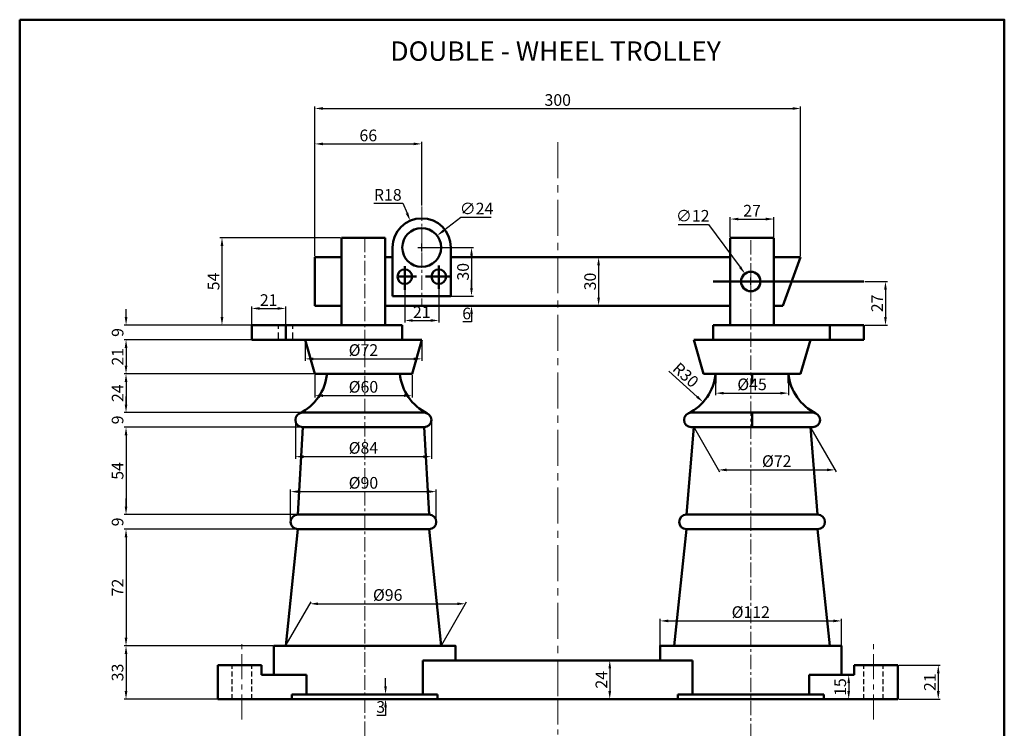
# Model space of a CAD drawing. Units: millimetres. Extents: x -25 to 583, y -116 to 549.
# Tile 2 of 2: x -25 to 583, y 111 to 549. Entities that reach past the tile are written whole.
import ezdxf

# ---------------------------------------------------------------- set-up
doc = ezdxf.new("R2010")
doc.units = ezdxf.units.MM
doc.header["$LTSCALE"] = 0.7
doc.linetypes.add('CENTER', pattern=[50.8, 31.75, -6.35, 6.35, -6.35])
doc.linetypes.add('HIDDEN', pattern=[9.525, 6.35, -3.175])
for name, color, linetype, lineweight in [('M-CNTR', 1, 'CENTER', 18), ('M-DIMS', 2, 'Continuous', 25), ('M-HIDN', 6, 'HIDDEN', 25), ('M-OUTL', 7, 'Continuous', 50), ('M-TEXT', 3, 'Continuous', 25), ('M-TTLB', 7, 'Continuous', 50)]:
    doc.layers.add(name, color=color, linetype=linetype, lineweight=lineweight)
doc.styles.get("Standard").update_dxf_attribs({"font": 'arial.ttf'})
doc.dimstyles.new('ISO-25', dxfattribs={"dimtxt": 7.2, "dimasz": 5, "dimexe": 1.25, "dimexo": 0.625, "dimtad": 1, "dimtoh": 1, "dimdec": 0, "dimtxsty": 'Standard', "dimcen": 2.5, "dimadec": 0, "dimazin": 0, "dimtfac": 1, "dimtdec": 0, "dimtofl": 0, "dimtmove": 0, "dimatfit": 3, "dimfxl": 1, "dimarcsym": 0})

# ---------------------------------------------------------------- blocks, each defined once
blk = doc.blocks.new('*D1')
at = {"layer": 'Defpoints', "color": 0, "ltscale": 0.4, "transparency": 16777216}
for p in [(327.7, 401.89), (327.7, 371.89), (332.69, 371.89)]:
    blk.add_point(p, dxfattribs=at)
at = {"layer": 'M-DIMS', "color": 0, "lineweight": -2, "ltscale": 0.4, "transparency": 16777216}
for p, q in [((328.33, 401.89), (333.94, 401.89)), ((332.69, 396.89), (332.69, 376.89)), ((328.33, 371.89), (333.94, 371.89))]:
    blk.add_line(p, q, dxfattribs=at)
at = {"layer": 'M-DIMS', "color": 0, "ltscale": 0.4, "transparency": 16777216}
for points in [[(331.85, 396.89), (333.52, 396.89), (332.69, 401.89)], [(331.85, 376.89), (333.52, 376.89), (332.69, 371.89)]]:
    blk.add_solid(points, dxfattribs=at)
at = {"layer": 'M-DIMS', "color": 0, "ltscale": 0.4, "transparency": 16777216, "insert": (328.38, 386.89), "char_height": 7.2, "attachment_point": 5, "rotation": 90}
blk.add_mtext('30', dxfattribs=at)
blk = doc.blocks.new('*D2')
at = {"layer": 'Defpoints', "color": 0, "ltscale": 0.4, "transparency": 16777216}
for p in [(250.43, 187.83), (139.45, 161.89), (235.45, 161.89)]:
    blk.add_point(p, dxfattribs=at)
at = {"layer": 'M-DIMS', "color": 0, "lineweight": -2, "ltscale": 0.4, "transparency": 16777216}
for p, q in [((139.81, 162.51), (155.15, 189.08)), ((235.81, 162.51), (251.15, 189.08)), ((159.43, 187.83), (245.43, 187.83))]:
    blk.add_line(p, q, dxfattribs=at)
at = {"layer": 'M-DIMS', "color": 0, "ltscale": 0.4, "transparency": 16777216}
for points in [[(159.43, 188.66), (159.43, 187), (154.43, 187.83)], [(245.43, 188.66), (245.43, 187), (250.43, 187.83)]]:
    blk.add_solid(points, dxfattribs=at)
at = {"layer": 'M-DIMS', "color": 0, "ltscale": 0.4, "transparency": 16777216, "insert": (202.43, 192.33), "char_height": 7.2, "attachment_point": 5}
blk.add_mtext('%%C96', dxfattribs=at)
blk = doc.blocks.new('*D3')
at = {"layer": 'Defpoints', "color": 0, "ltscale": 0.4, "transparency": 16777216}
for p in [(232.45, 257.09), (142.45, 238.39), (232.45, 238.39)]:
    blk.add_point(p, dxfattribs=at)
at = {"layer": 'M-DIMS', "color": 0, "lineweight": -2, "ltscale": 0.4, "transparency": 16777216}
for p, q in [((142.45, 239.01), (142.45, 258.34)), ((147.45, 257.09), (227.45, 257.09)), ((232.45, 239.01), (232.45, 258.34))]:
    blk.add_line(p, q, dxfattribs=at)
at = {"layer": 'M-DIMS', "color": 0, "ltscale": 0.4, "transparency": 16777216}
for points in [[(147.45, 257.93), (147.45, 256.26), (142.45, 257.09)], [(227.45, 257.93), (227.45, 256.26), (232.45, 257.09)]]:
    blk.add_solid(points, dxfattribs=at)
at = {"layer": 'M-DIMS', "color": 0, "ltscale": 0.4, "transparency": 16777216, "insert": (187.45, 261.6), "char_height": 7.2, "attachment_point": 5}
blk.add_mtext('%%C90', dxfattribs=at)
blk = doc.blocks.new('*D4')
at = {"layer": 'Defpoints', "color": 0, "ltscale": 0.4, "transparency": 16777216}
for p in [(145.45, 301.39), (229.45, 301.39), (229.45, 278.69)]:
    blk.add_point(p, dxfattribs=at)
at = {"layer": 'M-DIMS', "color": 0, "lineweight": -2, "ltscale": 0.4, "transparency": 16777216}
for p, q in [((145.45, 300.76), (145.45, 277.44)), ((229.45, 300.76), (229.45, 277.44)), ((150.45, 278.69), (224.45, 278.69))]:
    blk.add_line(p, q, dxfattribs=at)
at = {"layer": 'M-DIMS', "color": 0, "ltscale": 0.4, "transparency": 16777216}
for points in [[(150.45, 279.52), (150.45, 277.86), (145.45, 278.69)], [(224.45, 279.52), (224.45, 277.86), (229.45, 278.69)]]:
    blk.add_solid(points, dxfattribs=at)
at = {"layer": 'M-DIMS', "color": 0, "ltscale": 0.4, "transparency": 16777216, "insert": (187.45, 283.19), "char_height": 7.2, "attachment_point": 5}
blk.add_mtext('%%C84', dxfattribs=at)
blk = doc.blocks.new('*D5')
at = {"layer": 'Defpoints', "color": 0, "ltscale": 0.4, "transparency": 16777216}
for p in [(157.45, 329.89), (217.45, 329.89), (217.45, 316.39)]:
    blk.add_point(p, dxfattribs=at)
at = {"layer": 'M-DIMS', "color": 0, "lineweight": -2, "ltscale": 0.4, "transparency": 16777216}
for p, q in [((157.45, 329.26), (157.45, 315.14)), ((217.45, 329.26), (217.45, 315.14)), ((162.45, 316.39), (212.45, 316.39))]:
    blk.add_line(p, q, dxfattribs=at)
at = {"layer": 'M-DIMS', "color": 0, "ltscale": 0.4, "transparency": 16777216}
for points in [[(162.45, 317.22), (162.45, 315.55), (157.45, 316.39)], [(212.45, 317.22), (212.45, 315.55), (217.45, 316.39)]]:
    blk.add_solid(points, dxfattribs=at)
at = {"layer": 'M-DIMS', "color": 0, "ltscale": 0.4, "transparency": 16777216, "insert": (187.45, 320.89), "char_height": 7.2, "attachment_point": 5}
blk.add_mtext('%%C60', dxfattribs=at)
blk = doc.blocks.new('*D6')
at = {"layer": 'Defpoints', "color": 0, "ltscale": 0.4, "transparency": 16777216}
for p in [(151.45, 350.89), (223.45, 350.89), (223.45, 339.1)]:
    blk.add_point(p, dxfattribs=at)
at = {"layer": 'M-DIMS', "color": 0, "lineweight": -2, "ltscale": 0.4, "transparency": 16777216}
for p, q in [((151.45, 350.26), (151.45, 337.85)), ((223.45, 350.26), (223.45, 337.85)), ((156.45, 339.1), (218.45, 339.1))]:
    blk.add_line(p, q, dxfattribs=at)
at = {"layer": 'M-DIMS', "color": 0, "ltscale": 0.4, "transparency": 16777216}
for points in [[(156.45, 339.93), (156.45, 338.27), (151.45, 339.1)], [(218.45, 339.93), (218.45, 338.27), (223.45, 339.1)]]:
    blk.add_solid(points, dxfattribs=at)
at = {"layer": 'M-DIMS', "color": 0, "ltscale": 0.4, "transparency": 16777216, "insert": (187.45, 343.6), "char_height": 7.2, "attachment_point": 5}
blk.add_mtext('%%C72', dxfattribs=at)
blk = doc.blocks.new('*D7')
at = {"layer": 'Defpoints', "color": 0, "ltscale": 0.4, "transparency": 16777216}
for p in [(404.95, 329.89), (449.95, 329.89), (449.95, 317.91)]:
    blk.add_point(p, dxfattribs=at)
at = {"layer": 'M-DIMS', "color": 0, "lineweight": -2, "ltscale": 0.4, "transparency": 16777216}
for p, q in [((404.95, 329.26), (404.95, 316.66)), ((449.95, 329.26), (449.95, 316.66)), ((409.95, 317.91), (444.95, 317.91))]:
    blk.add_line(p, q, dxfattribs=at)
at = {"layer": 'M-DIMS', "color": 0, "ltscale": 0.4, "transparency": 16777216}
for points in [[(409.95, 318.75), (409.95, 317.08), (404.95, 317.91)], [(444.95, 318.75), (444.95, 317.08), (449.95, 317.91)]]:
    blk.add_solid(points, dxfattribs=at)
at = {"layer": 'M-DIMS', "color": 0, "ltscale": 0.4, "transparency": 16777216, "insert": (427.45, 322.41), "char_height": 7.2, "attachment_point": 5}
blk.add_mtext('%%C45', dxfattribs=at)
blk = doc.blocks.new('*D8')
at = {"layer": 'Defpoints', "color": 0, "ltscale": 0.4, "transparency": 16777216}
for p in [(391.45, 296.89), (463.45, 296.89), (478.68, 270.51)]:
    blk.add_point(p, dxfattribs=at)
at = {"layer": 'M-DIMS', "color": 0, "lineweight": -2, "ltscale": 0.4, "transparency": 16777216}
for p, q in [((391.81, 296.26), (407.4, 269.26)), ((463.81, 296.26), (479.4, 269.26)), ((411.68, 270.51), (473.68, 270.51))]:
    blk.add_line(p, q, dxfattribs=at)
at = {"layer": 'M-DIMS', "color": 0, "ltscale": 0.4, "transparency": 16777216}
for points in [[(411.68, 271.34), (411.68, 269.68), (406.68, 270.51)], [(473.68, 271.34), (473.68, 269.68), (478.68, 270.51)]]:
    blk.add_solid(points, dxfattribs=at)
at = {"layer": 'M-DIMS', "color": 0, "ltscale": 0.4, "transparency": 16777216, "insert": (442.68, 275.01), "char_height": 7.2, "attachment_point": 5}
blk.add_mtext('%%C72', dxfattribs=at)
blk = doc.blocks.new('*D9')
at = {"layer": 'Defpoints', "color": 0, "ltscale": 0.4, "transparency": 16777216}
for p in [(132.22, 161.89), (40.84, 128.89), (132.22, 128.89)]:
    blk.add_point(p, dxfattribs=at)
at = {"layer": 'M-DIMS', "color": 0, "lineweight": -2, "ltscale": 0.4, "transparency": 16777216}
for p, q in [((131.6, 161.89), (39.59, 161.89)), ((40.84, 156.89), (40.84, 133.89)), ((131.6, 128.89), (39.59, 128.89))]:
    blk.add_line(p, q, dxfattribs=at)
at = {"layer": 'M-DIMS', "color": 0, "ltscale": 0.4, "transparency": 16777216}
for points in [[(40, 156.89), (41.67, 156.89), (40.84, 161.89)], [(40, 133.89), (41.67, 133.89), (40.84, 128.89)]]:
    blk.add_solid(points, dxfattribs=at)
at = {"layer": 'M-DIMS', "color": 0, "ltscale": 0.4, "transparency": 16777216, "insert": (36.53, 145.39), "char_height": 7.2, "attachment_point": 5, "rotation": 90}
blk.add_mtext('33', dxfattribs=at)
blk = doc.blocks.new('*D10')
at = {"layer": 'Defpoints', "color": 0, "ltscale": 0.4, "transparency": 16777216}
for p in [(158.13, 233.89), (40.84, 161.89), (114.46, 161.89)]:
    blk.add_point(p, dxfattribs=at)
at = {"layer": 'M-DIMS', "color": 0, "lineweight": -2, "ltscale": 0.4, "transparency": 16777216}
for p, q in [((157.5, 233.89), (39.59, 233.89)), ((40.84, 228.89), (40.84, 166.89)), ((113.84, 161.89), (39.59, 161.89))]:
    blk.add_line(p, q, dxfattribs=at)
at = {"layer": 'M-DIMS', "color": 0, "ltscale": 0.4, "transparency": 16777216}
for points in [[(40, 228.89), (41.67, 228.89), (40.84, 233.89)], [(40, 166.89), (41.67, 166.89), (40.84, 161.89)]]:
    blk.add_solid(points, dxfattribs=at)
at = {"layer": 'M-DIMS', "color": 0, "ltscale": 0.4, "transparency": 16777216, "insert": (36.6, 197.89), "char_height": 7.2, "attachment_point": 5, "rotation": 90}
blk.add_mtext('72', dxfattribs=at)
blk = doc.blocks.new('*D11')
at = {"layer": 'Defpoints', "color": 0, "ltscale": 0.4, "transparency": 16777216}
for p in [(146.95, 242.89), (40.84, 233.89), (146.95, 233.89)]:
    blk.add_point(p, dxfattribs=at)
at = {"layer": 'M-DIMS', "color": 0, "lineweight": -2, "ltscale": 0.4, "transparency": 16777216}
for p, q in [((40.84, 247.89), (40.84, 252.89)), ((146.33, 242.89), (39.59, 242.89)), ((146.33, 233.89), (39.59, 233.89)), ((40.84, 228.89), (40.84, 223.89))]:
    blk.add_line(p, q, dxfattribs=at)
at = {"layer": 'M-DIMS', "color": 0, "ltscale": 0.4, "transparency": 16777216}
for points in [[(40, 247.89), (41.67, 247.89), (40.84, 242.89)], [(40, 228.89), (41.67, 228.89), (40.84, 233.89)]]:
    blk.add_solid(points, dxfattribs=at)
at = {"layer": 'M-DIMS', "color": 0, "ltscale": 0.4, "transparency": 16777216, "insert": (36.54, 238.39), "char_height": 7.2, "attachment_point": 5, "rotation": 90}
blk.add_mtext('9', dxfattribs=at)
blk = doc.blocks.new('*D12')
at = {"layer": 'Defpoints', "color": 0, "ltscale": 0.4, "transparency": 16777216}
for p in [(154.98, 296.89), (40.84, 242.89), (154.98, 242.89)]:
    blk.add_point(p, dxfattribs=at)
at = {"layer": 'M-DIMS', "color": 0, "lineweight": -2, "ltscale": 0.4, "transparency": 16777216}
for p, q in [((154.35, 296.89), (39.59, 296.89)), ((40.84, 291.89), (40.84, 247.89)), ((154.35, 242.89), (39.59, 242.89))]:
    blk.add_line(p, q, dxfattribs=at)
at = {"layer": 'M-DIMS', "color": 0, "ltscale": 0.4, "transparency": 16777216}
for points in [[(40, 291.89), (41.67, 291.89), (40.84, 296.89)], [(40, 247.89), (41.67, 247.89), (40.84, 242.89)]]:
    blk.add_solid(points, dxfattribs=at)
at = {"layer": 'M-DIMS', "color": 0, "ltscale": 0.4, "transparency": 16777216, "insert": (36.55, 269.89), "char_height": 7.2, "attachment_point": 5, "rotation": 90}
blk.add_mtext('54', dxfattribs=at)
blk = doc.blocks.new('*D13')
at = {"layer": 'Defpoints', "color": 0, "ltscale": 0.4, "transparency": 16777216}
for p in [(179.78, 305.89), (40.84, 296.89), (179.78, 296.89)]:
    blk.add_point(p, dxfattribs=at)
at = {"layer": 'M-DIMS', "color": 0, "lineweight": -2, "ltscale": 0.4, "transparency": 16777216}
for p, q in [((40.84, 310.89), (40.84, 315.89)), ((179.15, 305.89), (39.59, 305.89)), ((179.15, 296.89), (39.59, 296.89)), ((40.84, 291.89), (40.84, 286.89))]:
    blk.add_line(p, q, dxfattribs=at)
at = {"layer": 'M-DIMS', "color": 0, "ltscale": 0.4, "transparency": 16777216}
for points in [[(40, 310.89), (41.67, 310.89), (40.84, 305.89)], [(40, 291.89), (41.67, 291.89), (40.84, 296.89)]]:
    blk.add_solid(points, dxfattribs=at)
at = {"layer": 'M-DIMS', "color": 0, "ltscale": 0.4, "transparency": 16777216, "insert": (36.54, 301.39), "char_height": 7.2, "attachment_point": 5, "rotation": 90}
blk.add_mtext('9', dxfattribs=at)
blk = doc.blocks.new('*D14')
at = {"layer": 'Defpoints', "color": 0, "ltscale": 0.4, "transparency": 16777216}
for p in [(164.95, 329.89), (40.84, 305.89), (164.95, 305.89)]:
    blk.add_point(p, dxfattribs=at)
at = {"layer": 'M-DIMS', "color": 0, "lineweight": -2, "ltscale": 0.4, "transparency": 16777216}
for p, q in [((164.33, 329.89), (39.59, 329.89)), ((40.84, 324.89), (40.84, 310.89)), ((164.33, 305.89), (39.59, 305.89))]:
    blk.add_line(p, q, dxfattribs=at)
at = {"layer": 'M-DIMS', "color": 0, "ltscale": 0.4, "transparency": 16777216}
for points in [[(40, 324.89), (41.67, 324.89), (40.84, 329.89)], [(40, 310.89), (41.67, 310.89), (40.84, 305.89)]]:
    blk.add_solid(points, dxfattribs=at)
at = {"layer": 'M-DIMS', "color": 0, "ltscale": 0.4, "transparency": 16777216, "insert": (36.6, 317.89), "char_height": 7.2, "attachment_point": 5, "rotation": 90}
blk.add_mtext('24', dxfattribs=at)
blk = doc.blocks.new('*D15')
at = {"layer": 'Defpoints', "color": 0, "ltscale": 0.4, "transparency": 16777216}
for p in [(158.97, 350.89), (40.84, 329.89), (158.97, 329.89)]:
    blk.add_point(p, dxfattribs=at)
at = {"layer": 'M-DIMS', "color": 0, "lineweight": -2, "ltscale": 0.4, "transparency": 16777216}
for p, q in [((158.35, 350.89), (39.59, 350.89)), ((40.84, 345.89), (40.84, 334.89)), ((158.35, 329.89), (39.59, 329.89))]:
    blk.add_line(p, q, dxfattribs=at)
at = {"layer": 'M-DIMS', "color": 0, "ltscale": 0.4, "transparency": 16777216}
for points in [[(40, 345.89), (41.67, 345.89), (40.84, 350.89)], [(40, 334.89), (41.67, 334.89), (40.84, 329.89)]]:
    blk.add_solid(points, dxfattribs=at)
at = {"layer": 'M-DIMS', "color": 0, "ltscale": 0.4, "transparency": 16777216, "insert": (36.6, 340.39), "char_height": 7.2, "attachment_point": 5, "rotation": 90}
blk.add_mtext('21', dxfattribs=at)
blk = doc.blocks.new('*D16')
at = {"layer": 'Defpoints', "color": 0, "ltscale": 0.4, "transparency": 16777216}
for p in [(118.45, 359.89), (40.86, 350.89), (118.45, 350.89)]:
    blk.add_point(p, dxfattribs=at)
at = {"layer": 'M-DIMS', "color": 0, "lineweight": -2, "ltscale": 0.4, "transparency": 16777216}
for p, q in [((40.86, 364.89), (40.86, 369.89)), ((117.83, 359.89), (39.61, 359.89)), ((117.83, 350.89), (39.61, 350.89)), ((40.86, 345.89), (40.86, 340.89))]:
    blk.add_line(p, q, dxfattribs=at)
at = {"layer": 'M-DIMS', "color": 0, "ltscale": 0.4, "transparency": 16777216}
for points in [[(40.03, 364.89), (41.69, 364.89), (40.86, 359.89)], [(40.03, 345.89), (41.69, 345.89), (40.86, 350.89)]]:
    blk.add_solid(points, dxfattribs=at)
at = {"layer": 'M-DIMS', "color": 0, "ltscale": 0.4, "transparency": 16777216, "insert": (36.56, 355.39), "char_height": 7.2, "attachment_point": 5, "rotation": 90}
blk.add_mtext('9', dxfattribs=at)
blk = doc.blocks.new('*D17')
at = {"layer": 'Defpoints', "color": 0, "ltscale": 0.4, "transparency": 16777216}
for p in [(173.95, 413.89), (100.1, 359.89), (173.95, 359.89)]:
    blk.add_point(p, dxfattribs=at)
at = {"layer": 'M-DIMS', "color": 0, "lineweight": -2, "ltscale": 0.4, "transparency": 16777216}
for p, q in [((173.33, 413.89), (98.85, 413.89)), ((100.1, 408.89), (100.1, 364.89)), ((173.33, 359.89), (98.85, 359.89))]:
    blk.add_line(p, q, dxfattribs=at)
at = {"layer": 'M-DIMS', "color": 0, "ltscale": 0.4, "transparency": 16777216}
for points in [[(99.27, 408.89), (100.94, 408.89), (100.1, 413.89)], [(99.27, 364.89), (100.94, 364.89), (100.1, 359.89)]]:
    blk.add_solid(points, dxfattribs=at)
at = {"layer": 'M-DIMS', "color": 0, "ltscale": 0.4, "transparency": 16777216, "insert": (95.82, 386.89), "char_height": 7.2, "attachment_point": 5, "rotation": 90}
blk.add_mtext('54', dxfattribs=at)
blk = doc.blocks.new('*D18')
at = {"layer": 'Defpoints', "color": 0, "ltscale": 0.4, "transparency": 16777216}
for p in [(139.45, 370.24), (118.45, 359.89), (139.45, 359.89)]:
    blk.add_point(p, dxfattribs=at)
at = {"layer": 'M-DIMS', "color": 0, "lineweight": -2, "ltscale": 0.4, "transparency": 16777216}
for p, q in [((118.45, 360.51), (118.45, 371.49)), ((139.45, 360.51), (139.45, 371.49)), ((123.45, 370.24), (134.45, 370.24))]:
    blk.add_line(p, q, dxfattribs=at)
at = {"layer": 'M-DIMS', "color": 0, "ltscale": 0.4, "transparency": 16777216}
for points in [[(123.45, 371.07), (123.45, 369.4), (118.45, 370.24)], [(134.45, 371.07), (134.45, 369.4), (139.45, 370.24)]]:
    blk.add_solid(points, dxfattribs=at)
at = {"layer": 'M-DIMS', "color": 0, "ltscale": 0.4, "transparency": 16777216, "insert": (128.95, 374.48), "char_height": 7.2, "attachment_point": 5}
blk.add_mtext('21', dxfattribs=at)
blk = doc.blocks.new('*D19')
at = {"layer": 'Defpoints', "color": 0, "ltscale": 0.4, "transparency": 16777216}
for p in [(457.45, 493.74), (157.45, 401.89), (457.45, 401.89)]:
    blk.add_point(p, dxfattribs=at)
at = {"layer": 'M-DIMS', "color": 0, "lineweight": -2, "ltscale": 0.4, "transparency": 16777216}
for p, q in [((157.45, 402.51), (157.45, 494.99)), ((162.45, 493.74), (452.45, 493.74)), ((457.45, 402.51), (457.45, 494.99))]:
    blk.add_line(p, q, dxfattribs=at)
at = {"layer": 'M-DIMS', "color": 0, "ltscale": 0.4, "transparency": 16777216}
for points in [[(162.45, 494.57), (162.45, 492.91), (157.45, 493.74)], [(452.45, 494.57), (452.45, 492.91), (457.45, 493.74)]]:
    blk.add_solid(points, dxfattribs=at)
at = {"layer": 'M-DIMS', "color": 0, "ltscale": 0.4, "transparency": 16777216, "insert": (307.45, 498.04), "char_height": 7.2, "attachment_point": 5}
blk.add_mtext('300', dxfattribs=at)
blk = doc.blocks.new('*D20')
at = {"layer": 'Defpoints', "color": 0, "ltscale": 0.4, "transparency": 16777216}
for p in [(223.45, 471.87), (157.45, 448.75), (223.45, 433.22)]:
    blk.add_point(p, dxfattribs=at)
at = {"layer": 'M-DIMS', "color": 0, "lineweight": -2, "ltscale": 0.4, "transparency": 16777216}
for p, q in [((157.45, 449.38), (157.45, 473.12)), ((162.45, 471.87), (218.45, 471.87)), ((223.45, 433.84), (223.45, 473.12))]:
    blk.add_line(p, q, dxfattribs=at)
at = {"layer": 'M-DIMS', "color": 0, "ltscale": 0.4, "transparency": 16777216}
for points in [[(162.45, 472.7), (162.45, 471.03), (157.45, 471.87)], [(218.45, 472.7), (218.45, 471.03), (223.45, 471.87)]]:
    blk.add_solid(points, dxfattribs=at)
at = {"layer": 'M-DIMS', "color": 0, "ltscale": 0.4, "transparency": 16777216, "insert": (190.45, 476.17), "char_height": 7.2, "attachment_point": 5}
blk.add_mtext('66', dxfattribs=at)
blk = doc.blocks.new('*D21')
at = {"layer": 'Defpoints', "color": 0, "ltscale": 0.4, "transparency": 16777216}
for p in [(237.7, 377.89), (237.7, 371.89), (254.2, 371.89)]:
    blk.add_point(p, dxfattribs=at)
at = {"layer": 'M-DIMS', "color": 0, "lineweight": -2, "ltscale": 0.4, "transparency": 16777216}
for p, q in [((254.2, 382.89), (254.2, 387.89)), ((238.33, 377.89), (255.45, 377.89)), ((238.33, 371.89), (255.45, 371.89)), ((254.2, 366.89), (254.2, 361.89)), ((254.2, 361.89), (248.82, 361.89))]:
    blk.add_line(p, q, dxfattribs=at)
at = {"layer": 'M-DIMS', "color": 0, "ltscale": 0.4, "transparency": 16777216}
for points in [[(253.37, 382.89), (255.03, 382.89), (254.2, 377.89)], [(253.37, 366.89), (255.03, 366.89), (254.2, 371.89)]]:
    blk.add_solid(points, dxfattribs=at)
at = {"layer": 'M-DIMS', "color": 0, "ltscale": 0.4, "transparency": 16777216, "insert": (251.2, 366.19), "char_height": 7.2, "attachment_point": 5}
blk.add_mtext('6', dxfattribs=at)
blk = doc.blocks.new('*D22')
at = {"layer": 'Defpoints', "color": 0, "ltscale": 0.4, "transparency": 16777216}
for p in [(223.45, 407.89), (223.45, 377.89), (254.2, 377.89)]:
    blk.add_point(p, dxfattribs=at)
at = {"layer": 'M-DIMS', "color": 0, "lineweight": -2, "ltscale": 0.4, "transparency": 16777216}
for p, q in [((224.08, 407.89), (255.45, 407.89)), ((254.2, 402.89), (254.2, 382.89)), ((224.08, 377.89), (255.45, 377.89))]:
    blk.add_line(p, q, dxfattribs=at)
at = {"layer": 'M-DIMS', "color": 0, "ltscale": 0.4, "transparency": 16777216}
for points in [[(253.37, 402.89), (255.03, 402.89), (254.2, 407.89)], [(253.37, 382.89), (255.03, 382.89), (254.2, 377.89)]]:
    blk.add_solid(points, dxfattribs=at)
at = {"layer": 'M-DIMS', "color": 0, "ltscale": 0.4, "transparency": 16777216, "insert": (249.9, 392.89), "char_height": 7.2, "attachment_point": 5, "rotation": 90}
blk.add_mtext('30', dxfattribs=at)
blk = doc.blocks.new('*D23')
at = {"layer": 'Defpoints', "color": 0, "ltscale": 0.4, "transparency": 16777216}
for p in [(212.95, 389.89), (233.95, 389.89), (233.95, 362.81)]:
    blk.add_point(p, dxfattribs=at)
at = {"layer": 'M-DIMS', "color": 0, "lineweight": -2, "ltscale": 0.4, "transparency": 16777216}
for p, q in [((212.95, 389.26), (212.95, 361.56)), ((233.95, 389.26), (233.95, 361.56)), ((217.95, 362.81), (228.95, 362.81))]:
    blk.add_line(p, q, dxfattribs=at)
at = {"layer": 'M-DIMS', "color": 0, "ltscale": 0.4, "transparency": 16777216}
for points in [[(217.95, 363.64), (217.95, 361.98), (212.95, 362.81)], [(228.95, 363.64), (228.95, 361.98), (233.95, 362.81)]]:
    blk.add_solid(points, dxfattribs=at)
at = {"layer": 'M-DIMS', "color": 0, "ltscale": 0.4, "transparency": 16777216, "insert": (223.45, 367.05), "char_height": 7.2, "attachment_point": 5}
blk.add_mtext('21', dxfattribs=at)
blk = doc.blocks.new('*D24')
at = {"layer": 'Defpoints', "color": 0, "ltscale": 0.4, "transparency": 16777216}
for p in [(232.96, 415.2), (213.94, 400.57)]:
    blk.add_point(p, dxfattribs=at)
at = {"layer": 'M-DIMS', "color": 0, "lineweight": -2, "ltscale": 0.4, "transparency": 16777216}
for p, q in [((247.63, 426.48), (236.93, 418.25)), ((266.37, 426.48), (247.63, 426.48)), ((220.95, 407.89), (225.95, 407.89)), ((223.45, 405.39), (223.45, 410.39))]:
    blk.add_line(p, q, dxfattribs=at)
at = {"layer": 'M-DIMS', "color": 0, "ltscale": 0.4, "transparency": 16777216}
blk.add_solid([(236.42, 418.91), (237.43, 417.59), (232.96, 415.2)], dxfattribs=at)
at = {"layer": 'M-DIMS', "color": 0, "ltscale": 0.4, "transparency": 16777216, "insert": (257.31, 430.98), "char_height": 7.2, "attachment_point": 5}
blk.add_mtext('∅24', dxfattribs=at)
blk = doc.blocks.new('*D25')
at = {"layer": 'Defpoints', "color": 0, "ltscale": 0.4, "transparency": 16777216}
for p in [(216.34, 424.42), (223.45, 407.89)]:
    blk.add_point(p, dxfattribs=at)
at = {"layer": 'M-DIMS', "color": 0, "lineweight": -2, "ltscale": 0.4, "transparency": 16777216}
for p, q in [((193.88, 435.17), (211.72, 435.17)), ((211.72, 435.17), (214.37, 429.02)), ((220.95, 407.89), (225.95, 407.89)), ((223.45, 405.39), (223.45, 410.39))]:
    blk.add_line(p, q, dxfattribs=at)
at = {"layer": 'M-DIMS', "color": 0, "ltscale": 0.4, "transparency": 16777216}
blk.add_solid([(215.13, 429.35), (213.6, 428.69), (216.34, 424.42)], dxfattribs=at)
at = {"layer": 'M-DIMS', "color": 0, "ltscale": 0.4, "transparency": 16777216, "insert": (202.49, 439.47), "char_height": 7.2, "attachment_point": 5}
blk.add_mtext('R18', dxfattribs=at)
blk = doc.blocks.new('*D26')
at = {"layer": 'Defpoints', "color": 0, "ltscale": 0.4, "transparency": 16777216}
for p in [(496.45, 386.89), (496.45, 359.89), (509.86, 359.89)]:
    blk.add_point(p, dxfattribs=at)
at = {"layer": 'M-DIMS', "color": 0, "lineweight": -2, "ltscale": 0.4, "transparency": 16777216}
for p, q in [((497.08, 386.89), (511.11, 386.89)), ((509.86, 381.89), (509.86, 364.89)), ((497.08, 359.89), (511.11, 359.89))]:
    blk.add_line(p, q, dxfattribs=at)
at = {"layer": 'M-DIMS', "color": 0, "ltscale": 0.4, "transparency": 16777216}
for points in [[(509.02, 381.89), (510.69, 381.89), (509.86, 386.89)], [(509.02, 364.89), (510.69, 364.89), (509.86, 359.89)]]:
    blk.add_solid(points, dxfattribs=at)
at = {"layer": 'M-DIMS', "color": 0, "ltscale": 0.4, "transparency": 16777216, "insert": (505.62, 373.39), "char_height": 7.2, "attachment_point": 5, "rotation": 90}
blk.add_mtext('27', dxfattribs=at)
blk = doc.blocks.new('*D27')
at = {"layer": 'Defpoints', "color": 0, "ltscale": 0.4, "transparency": 16777216}
for p in [(440.95, 425.45), (413.95, 413.89), (440.95, 413.89)]:
    blk.add_point(p, dxfattribs=at)
at = {"layer": 'M-DIMS', "color": 0, "lineweight": -2, "ltscale": 0.4, "transparency": 16777216}
for p, q in [((413.95, 414.51), (413.95, 426.7)), ((440.95, 414.51), (440.95, 426.7)), ((418.95, 425.45), (435.95, 425.45))]:
    blk.add_line(p, q, dxfattribs=at)
at = {"layer": 'M-DIMS', "color": 0, "ltscale": 0.4, "transparency": 16777216}
for points in [[(418.95, 426.28), (418.95, 424.62), (413.95, 425.45)], [(435.95, 426.28), (435.95, 424.62), (440.95, 425.45)]]:
    blk.add_solid(points, dxfattribs=at)
at = {"layer": 'M-DIMS', "color": 0, "ltscale": 0.4, "transparency": 16777216, "insert": (427.45, 429.69), "char_height": 7.2, "attachment_point": 5}
blk.add_mtext('27', dxfattribs=at)
blk = doc.blocks.new('*D28')
at = {"layer": 'Defpoints', "color": 0, "ltscale": 0.4, "transparency": 16777216}
for p in [(374.67, 332.79), (397.22, 312.37)]:
    blk.add_point(p, dxfattribs=at)
at = {"layer": 'M-DIMS', "color": 0, "lineweight": -2, "ltscale": 0.4, "transparency": 16777216}
blk.add_line((376.14, 331.45), (393.51, 315.73), dxfattribs=at)
at = {"layer": 'M-DIMS', "color": 0, "ltscale": 0.4, "transparency": 16777216}
blk.add_solid([(394.07, 316.34), (392.96, 315.11), (397.22, 312.37)], dxfattribs=at)
at = {"layer": 'M-DIMS', "color": 0, "ltscale": 0.4, "transparency": 16777216, "insert": (385.86, 328.46), "char_height": 7.2, "attachment_point": 5, "rotation": 317.84948}
blk.add_mtext('R30', dxfattribs=at)
blk = doc.blocks.new('*D29')
at = {"layer": 'Defpoints', "color": 0, "ltscale": 0.4, "transparency": 16777216}
for p in [(423.09, 391.7), (430.27, 382.08)]:
    blk.add_point(p, dxfattribs=at)
at = {"layer": 'M-DIMS', "color": 0, "lineweight": -2, "ltscale": 0.4, "transparency": 16777216}
for p, q in [((381.8, 422.01), (400.5, 422.01)), ((400.5, 422.01), (420.11, 395.7)), ((426.68, 384.39), (426.68, 389.39)), ((424.18, 386.89), (429.18, 386.89))]:
    blk.add_line(p, q, dxfattribs=at)
at = {"layer": 'M-DIMS', "color": 0, "ltscale": 0.4, "transparency": 16777216}
blk.add_solid([(420.77, 396.2), (419.44, 395.21), (423.09, 391.7)], dxfattribs=at)
at = {"layer": 'M-DIMS', "color": 0, "ltscale": 0.4, "transparency": 16777216, "insert": (390.83, 426.51), "char_height": 7.2, "attachment_point": 5}
blk.add_mtext('∅12', dxfattribs=at)
blk = doc.blocks.new('*D30')
at = {"layer": 'Defpoints', "color": 0, "ltscale": 0.4, "transparency": 16777216}
for p in [(482.68, 177.24), (370.68, 161.89), (482.68, 161.89)]:
    blk.add_point(p, dxfattribs=at)
at = {"layer": 'M-DIMS', "color": 0, "lineweight": -2, "ltscale": 0.4, "transparency": 16777216}
for p, q in [((370.68, 162.51), (370.68, 178.49)), ((375.68, 177.24), (477.68, 177.24)), ((482.68, 162.51), (482.68, 178.49))]:
    blk.add_line(p, q, dxfattribs=at)
at = {"layer": 'M-DIMS', "color": 0, "ltscale": 0.4, "transparency": 16777216}
for points in [[(375.68, 178.08), (375.68, 176.41), (370.68, 177.24)], [(477.68, 178.08), (477.68, 176.41), (482.68, 177.24)]]:
    blk.add_solid(points, dxfattribs=at)
at = {"layer": 'M-DIMS', "color": 0, "ltscale": 0.4, "transparency": 16777216, "insert": (426.68, 181.74), "char_height": 7.2, "attachment_point": 5}
blk.add_mtext('%%C112', dxfattribs=at)
blk = doc.blocks.new('*D31')
at = {"layer": 'Defpoints', "color": 0, "ltscale": 0.4, "transparency": 16777216}
for p in [(517.45, 149.89), (517.45, 128.89), (542.46, 128.89)]:
    blk.add_point(p, dxfattribs=at)
at = {"layer": 'M-DIMS', "color": 0, "lineweight": -2, "ltscale": 0.4, "transparency": 16777216}
for p, q in [((518.08, 149.89), (543.71, 149.89)), ((542.46, 144.89), (542.46, 133.89)), ((518.08, 128.89), (543.71, 128.89))]:
    blk.add_line(p, q, dxfattribs=at)
at = {"layer": 'M-DIMS', "color": 0, "ltscale": 0.4, "transparency": 16777216}
for points in [[(541.62, 144.89), (543.29, 144.89), (542.46, 149.89)], [(541.62, 133.89), (543.29, 133.89), (542.46, 128.89)]]:
    blk.add_solid(points, dxfattribs=at)
at = {"layer": 'M-DIMS', "color": 0, "ltscale": 0.4, "transparency": 16777216, "insert": (538.22, 139.39), "char_height": 7.2, "attachment_point": 5, "rotation": 90}
blk.add_mtext('21', dxfattribs=at)
blk = doc.blocks.new('*D32')
at = {"layer": 'Defpoints', "color": 0, "ltscale": 0.7, "transparency": 16777216}
for p in [(486.74, 143.89), (486.74, 128.89), (487.14, 128.89)]:
    blk.add_point(p, dxfattribs=at)
at = {"layer": 'M-DIMS', "color": 0, "lineweight": -2, "ltscale": 0.7, "transparency": 16777216}
for p, q in [((487.36, 143.89), (488.39, 143.89)), ((487.14, 138.89), (487.14, 133.89)), ((487.36, 128.89), (488.39, 128.89))]:
    blk.add_line(p, q, dxfattribs=at)
at = {"layer": 'M-DIMS', "color": 0, "ltscale": 0.7, "transparency": 16777216}
for points in [[(486.31, 138.89), (487.97, 138.89), (487.14, 143.89)], [(486.31, 133.89), (487.97, 133.89), (487.14, 128.89)]]:
    blk.add_solid(points, dxfattribs=at)
at = {"layer": 'M-DIMS', "color": 0, "ltscale": 0.7, "transparency": 16777216, "insert": (482.84, 136.39), "char_height": 7.2, "attachment_point": 5, "rotation": 90}
blk.add_mtext('15', dxfattribs=at)
blk = doc.blocks.new('*D33')
at = {"layer": 'Defpoints', "color": 0, "ltscale": 0.7, "transparency": 16777216}
for p in [(339.58, 152.89), (339.58, 128.89), (339.58, 128.89)]:
    blk.add_point(p, dxfattribs=at)
at = {"layer": 'M-DIMS', "color": 0, "lineweight": -2, "ltscale": 0.7, "transparency": 16777216}
for p, q in [((340.2, 152.89), (340.83, 152.89)), ((339.58, 147.89), (339.58, 133.89)), ((340.2, 128.89), (340.83, 128.89))]:
    blk.add_line(p, q, dxfattribs=at)
at = {"layer": 'M-DIMS', "color": 0, "ltscale": 0.7, "transparency": 16777216}
for points in [[(338.74, 147.89), (340.41, 147.89), (339.58, 152.89)], [(338.74, 133.89), (340.41, 133.89), (339.58, 128.89)]]:
    blk.add_solid(points, dxfattribs=at)
at = {"layer": 'M-DIMS', "color": 0, "ltscale": 0.7, "transparency": 16777216, "insert": (335.34, 140.89), "char_height": 7.2, "attachment_point": 5, "rotation": 90}
blk.add_mtext('24', dxfattribs=at)
blk = doc.blocks.new('*D35')
at = {"layer": 'Defpoints', "color": 0, "ltscale": 0.7, "transparency": 16777216}
for p in [(201.1, 131.89), (201.1, 128.89), (201.1, 128.89)]:
    blk.add_point(p, dxfattribs=at)
at = {"layer": 'M-DIMS', "color": 0, "lineweight": -2, "ltscale": 0.7, "transparency": 16777216}
for p, q in [((201.1, 136.89), (201.1, 141.89)), ((201.73, 131.89), (202.35, 131.89)), ((201.73, 128.89), (202.35, 128.89)), ((201.1, 123.89), (201.1, 118.89)), ((201.1, 118.89), (195.76, 118.89))]:
    blk.add_line(p, q, dxfattribs=at)
at = {"layer": 'M-DIMS', "color": 0, "ltscale": 0.7, "transparency": 16777216}
for points in [[(200.27, 136.89), (201.93, 136.89), (201.1, 131.89)], [(200.27, 123.89), (201.93, 123.89), (201.1, 128.89)]]:
    blk.add_solid(points, dxfattribs=at)
at = {"layer": 'M-DIMS', "color": 0, "ltscale": 0.7, "transparency": 16777216, "insert": (198.12, 123.19), "char_height": 7.2, "attachment_point": 5}
blk.add_mtext('3', dxfattribs=at)

msp = doc.modelspace()

# ---------------------------------------------------------------- linework, layer by layer
at = {"layer": 'M-CNTR'}
msp.add_line((307.45, 472.96), (307.45, 128.89), dxfattribs=at)
at = {"layer": 'M-CNTR', "ltscale": 0.4}
for p, q in [((223.45, 433.22), (223.45, 371.89)), ((188.22, 413.89), (188.22, -85.81)), ((426.68, 412.37), (426.68, -69.19))]:
    msp.add_line(p, q, dxfattribs=at)
at = {"layer": 'M-CNTR', "ltscale": 0.7}
for p, q in [((112.45, 116.29), (112.45, 164.68)), ((502.45, 116.29), (502.45, 164.68)), ((307.45, 128.89), (307.45, -67.34))]:
    msp.add_line(p, q, dxfattribs=at)
at = {"layer": 'M-HIDN'}
for p, q in [((134.95, 350.89), (134.95, 359.89)), ((143.95, 350.89), (143.95, 359.89))]:
    msp.add_line(p, q, dxfattribs=at)
at = {"layer": 'M-HIDN', "ltscale": 0.7}
for p, q in [((106.45, 128.89), (106.45, 149.89)), ((118.45, 128.89), (118.45, 149.89)), ((496.45, 128.89), (496.45, 149.89)), ((508.45, 128.89), (508.45, 149.89))]:
    msp.add_line(p, q, dxfattribs=at)
at = {"layer": 'M-OUTL'}
for p, q in [((173.95, 413.89), (200.95, 413.89)), ((173.95, 359.89), (173.95, 413.89)), ((200.95, 413.89), (200.95, 359.89)), ((440.95, 413.89), (413.95, 413.89)), ((413.95, 413.89), (413.95, 359.89)), ((440.95, 359.89), (440.95, 413.89)), ((200.95, 401.89), (205.45, 401.89)), ((241.45, 401.89), (413.95, 401.89)), ((496.45, 386.89), (403.45, 386.89)), ((200.95, 371.89), (413.95, 371.89)), ((118.45, 350.89), (118.45, 359.89)), ((118.45, 359.89), (211.45, 359.89)), ((139.45, 350.89), (139.45, 359.89)), ((200.95, 359.89), (173.95, 359.89)), ((211.45, 359.89), (211.45, 350.89)), ((496.45, 359.89), (403.45, 359.89)), ((403.45, 359.89), (403.45, 350.89)), ((413.95, 359.89), (440.95, 359.89)), ((475.45, 350.89), (475.45, 359.89)), ((496.45, 350.89), (496.45, 359.89)), ((187.45, 350.89), (118.45, 350.89)), ((151.45, 350.89), (223.45, 350.89)), ((151.45, 350.89), (157.45, 329.89)), ((223.45, 350.89), (217.45, 329.89)), ((463.45, 350.89), (391.45, 350.89)), ((391.45, 350.89), (397.45, 329.89)), ((427.45, 350.89), (496.45, 350.89)), ((463.45, 350.89), (457.45, 329.89)), ((157.45, 329.89), (217.45, 329.89)), ((157.45, 329.89), (217.45, 329.89)), ((457.45, 329.89), (397.45, 329.89)), ((457.45, 329.89), (397.45, 329.89)), ((404.95, 329.89), (404.95, 324.1)), ((427.45, 329.89), (427.45, 324.1)), ((449.95, 329.89), (449.95, 324.1)), ((149.95, 305.89), (224.95, 305.89)), ((464.95, 305.89), (389.95, 305.89)), ((146.95, 242.89), (149.95, 296.89)), ((224.95, 296.89), (149.95, 296.89)), ((227.95, 242.89), (224.95, 296.94)), ((389.95, 296.89), (464.95, 296.89)), ((146.95, 242.89), (227.95, 242.89)), ((467.95, 242.89), (386.95, 242.89)), ((139.45, 161.89), (146.95, 233.89)), ((227.95, 233.89), (146.95, 233.89)), ((223.45, 233.89), (151.45, 233.89)), ((187.45, 233.89), (223.45, 233.89)), ((235.45, 161.89), (227.95, 233.89)), ((379.45, 161.89), (386.95, 233.89)), ((386.95, 233.89), (467.95, 233.89)), ((391.45, 233.89), (463.45, 233.89)), ((427.45, 233.89), (391.45, 233.89)), ((475.45, 161.89), (467.95, 233.89)), ((132.22, 161.89), (244.22, 161.89)), ((139.45, 161.89), (235.45, 161.89)), ((390.68, 152.89), (224.22, 152.89)), ((97.45, 149.89), (97.45, 128.89)), ((97.45, 128.89), (97.45, 149.89)), ((517.45, 128.89), (517.45, 149.89)), ((97.45, 128.89), (517.45, 128.89))]:
    msp.add_line(p, q, dxfattribs=at)
at = {"layer": 'M-OUTL', "ltscale": 0.4}
for p, q in [((205.45, 407.89), (205.45, 377.89)), ((241.45, 407.89), (241.45, 377.89)), ((157.45, 401.89), (157.45, 371.89)), ((173.95, 401.89), (157.45, 401.89)), ((440.95, 401.89), (457.45, 401.89)), ((457.45, 401.89), (446.41, 371.89)), ((212.95, 396.35), (212.95, 381.77)), ((233.95, 396.67), (233.95, 382.34)), ((208.45, 389.89), (220.17, 389.89)), ((241.45, 389.89), (225.7, 389.89)), ((205.45, 377.89), (211.45, 377.89)), ((211.45, 377.89), (235.45, 377.89)), ((241.45, 377.89), (233.95, 377.89)), ((157.45, 371.89), (173.95, 371.89)), ((200.95, 371.89), (307.45, 371.89)), ((440.95, 371.89), (446.41, 371.89)), ((427.45, 305.89), (427.45, 296.89)), ((386.95, 242.89), (391.45, 296.89)), ((467.95, 242.89), (463.45, 296.89)), ((224.22, 152.89), (224.22, 131.89)), ((390.68, 152.89), (390.68, 131.89)), ((97.45, 149.89), (124.45, 149.89)), ((124.45, 149.89), (124.45, 143.89)), ((517.45, 149.89), (490.45, 149.89)), ((490.45, 149.89), (490.45, 143.89)), ((124.45, 143.89), (152.22, 143.89)), ((152.22, 143.89), (152.22, 131.89)), ((462.68, 143.89), (462.68, 131.89)), ((490.45, 143.89), (462.68, 143.89)), ((482.68, 128.89), (517.45, 128.89))]:
    msp.add_line(p, q, dxfattribs=at)
at = {"layer": 'M-OUTL', "ltscale": 0.7}
for p, q in [((143.22, 128.89), (143.22, 131.89)), ((143.22, 131.89), (233.22, 131.89)), ((233.22, 131.89), (233.22, 128.89)), ((471.68, 131.89), (381.68, 131.89)), ((381.68, 131.89), (381.68, 128.89)), ((471.68, 128.89), (471.68, 131.89))]:
    msp.add_line(p, q, dxfattribs=at)
at = {"layer": 'M-OUTL'}
for points in [[(244.22, 152.89), (244.22, 161.89), (132.22, 161.89), (132.22, 143.89)], [(370.68, 152.89), (370.68, 161.89), (482.68, 161.89), (482.68, 143.89)], [(132.22, 128.89), (244.22, 128.89)]]:
    msp.add_lwpolyline(points, dxfattribs=at)
at = {"layer": 'M-OUTL', "ltscale": 0.4}
for centre, radius in [((223.45, 407.89), 12), ((212.95, 389.89), 4.5), ((233.95, 389.89), 4.5), ((426.68, 386.89), 6)]:
    msp.add_circle(centre, radius, dxfattribs=at)
msp.add_arc((223.45, 407.89), 18, 0, 180, dxfattribs=at)
at = {"layer": 'M-OUTL'}
for centre, radius, start, end in [((134.67, 332.79), 30.42, 295.98268, 354.528), ((240.24, 332.79), 30.42, 185.472, 244.01732), ((374.67, 332.79), 30.42, 295.98268, 354.528), ((480.24, 332.79), 30.42, 185.472, 244.01732), ((149.95, 301.39), 4.5, 90, 270), ((224.95, 301.39), 4.5, 270, 90), ((389.95, 301.39), 4.5, 90, 270), ((464.95, 301.39), 4.5, 270, 90), ((146.95, 238.39), 4.5, 90, 270), ((227.95, 238.39), 4.5, 270, 90), ((386.95, 238.39), 4.5, 90, 270), ((467.95, 238.39), 4.5, 270, 90)]:
    msp.add_arc(centre, radius, start, end, dxfattribs=at)
at = {"layer": 'M-TTLB', "ltscale": 0.7}
msp.add_lwpolyline([(-24.83, 548.59), (583.23, 548.59), (583.23, -116), (-24.83, -116)], close=True, dxfattribs=at)

# ---------------------------------------------------------------- texts
at = {"layer": 'M-TEXT', "ltscale": 0.7, "insert": (204.07, 535.18), "char_height": 12, "attachment_point": 1}
msp.add_mtext_dynamic_manual_height_columns('DOUBLE - WHEEL TROLLEY', width=261.1427, gutter_width=12.5, heights=[0], dxfattribs=at)

# ---------------------------------------------------------------- dimensions: what is measured, and where the dimension line sits
at = {"layer": 'M-DIMS', "ltscale": 0.4}
for base, p1, p2, picture, middle in [((457.45, 493.74), (157.45, 401.89), (457.45, 401.89), '*D19', (307.45, 498.04)), ((223.45, 471.87), (157.45, 448.75), (223.45, 433.22), '*D20', (190.45, 476.17)), ((440.95, 425.45), (413.95, 413.89), (440.95, 413.89), '*D27', (427.45, 429.69)), ((233.95, 362.81), (212.95, 389.89), (233.95, 389.89), '*D23', (223.45, 367.05)), ((139.45, 370.24), (118.45, 359.89), (139.45, 359.89), '*D18', (128.95, 374.48))]:
    dim = msp.add_linear_dim(base=base, p1=p1, p2=p2, dimstyle='ISO-25', override={"dimclrd": 0, "dimclre": 0, "dimclrt": 0}, dxfattribs=at)
    dim.commit()
    dim.dimension.update_dxf_attribs({"geometry": picture, "text_midpoint": middle})
for center, mpoint, picture, middle in [((223.45, 407.89), (216.34, 424.42), '*D25', (202.49, 435.17)), ((374.67, 332.79), (397.22, 312.37), '*D28', (382.98, 325.26))]:
    dim = msp.add_radius_dim(center=center, mpoint=mpoint, dimstyle='ISO-25', override={"dimclrd": 0, "dimclre": 0, "dimclrt": 0}, dxfattribs=at)
    dim.commit()
    dim.dimension.update_dxf_attribs({"geometry": picture, "text_midpoint": middle, "dimtype": 164})
for p1, p2, picture, middle in [((213.94, 400.57), (232.96, 415.2), '*D24', (257.31, 426.48)), ((430.27, 382.08), (423.09, 391.7), '*D29', (390.83, 422.01))]:
    dim = msp.add_diameter_dim_2p(p1=p1, p2=p2, dimstyle='ISO-25', override={"dimclrd": 0, "dimclre": 0, "dimclrt": 0}, dxfattribs=at)
    dim.commit()
    dim.dimension.update_dxf_attribs({"geometry": picture, "text_midpoint": middle, "dimtype": 163})
for base, p1, p2, picture, middle in [((100.1, 359.89), (173.95, 413.89), (173.95, 359.89), '*D17', (95.82, 386.89)), ((254.2, 377.89), (223.45, 407.89), (223.45, 377.89), '*D22', (249.9, 392.89)), ((332.69, 371.89), (327.7, 401.89), (327.7, 371.89), '*D1', (328.38, 386.89)), ((254.2, 371.89), (237.7, 377.89), (237.7, 371.89), '*D21', (251.2, 366.19)), ((509.86, 359.89), (496.45, 386.89), (496.45, 359.89), '*D26', (505.62, 373.39)), ((40.86, 350.89), (118.45, 359.89), (118.45, 350.89), '*D16', (36.56, 355.39)), ((40.84, 329.89), (158.97, 350.89), (158.97, 329.89), '*D15', (36.6, 340.39)), ((40.84, 305.89), (164.95, 329.89), (164.95, 305.89), '*D14', (36.6, 317.89)), ((40.84, 296.89), (179.78, 305.89), (179.78, 296.89), '*D13', (36.54, 301.39)), ((40.84, 242.89), (154.98, 296.89), (154.98, 242.89), '*D12', (36.55, 269.89)), ((40.84, 233.89), (146.95, 242.89), (146.95, 233.89), '*D11', (36.54, 238.39)), ((40.84, 161.89), (158.13, 233.89), (114.46, 161.89), '*D10', (36.6, 197.89)), ((40.84, 128.89), (132.22, 161.89), (132.22, 128.89), '*D9', (36.53, 145.39)), ((542.46, 128.89), (517.45, 149.89), (517.45, 128.89), '*D31', (538.22, 139.39))]:
    dim = msp.add_linear_dim(base=base, p1=p1, p2=p2, angle=90, dimstyle='ISO-25', override={"dimclrd": 0, "dimclre": 0, "dimclrt": 0}, dxfattribs=at)
    dim.commit()
    dim.dimension.update_dxf_attribs({"geometry": picture, "text_midpoint": middle})
for base, p1, p2, picture, middle in [((223.45, 339.1), (151.45, 350.89), (223.45, 350.89), '*D6', (187.45, 343.6)), ((217.45, 316.39), (157.45, 329.89), (217.45, 329.89), '*D5', (187.45, 320.89)), ((449.95, 317.91), (404.95, 329.89), (449.95, 329.89), '*D7', (427.45, 322.41)), ((229.45, 278.69), (145.45, 301.39), (229.45, 301.39), '*D4', (187.45, 283.19)), ((478.68, 270.51), (391.45, 296.89), (463.45, 296.89), '*D8', (442.68, 275.01)), ((232.45, 257.09), (142.45, 238.39), (232.45, 238.39), '*D3', (187.45, 261.6)), ((250.43, 187.83), (139.45, 161.89), (235.45, 161.89), '*D2', (202.43, 192.33)), ((482.68, 177.24), (370.68, 161.89), (482.68, 161.89), '*D30', (426.68, 181.74))]:
    dim = msp.add_linear_dim(base=base, p1=p1, p2=p2, text='%%C<>', dimstyle='ISO-25', override={"dimclrd": 0, "dimclre": 0, "dimclrt": 0}, dxfattribs=at)
    dim.commit()
    dim.dimension.update_dxf_attribs({"geometry": picture, "text_midpoint": middle})
at = {"layer": 'M-DIMS', "ltscale": 0.7}
for base, p1, p2, picture, middle in [((339.58, 128.89), (339.58, 152.89), (339.58, 128.89), '*D33', (335.34, 140.89)), ((201.1, 128.89), (201.1, 131.89), (201.1, 128.89), '*D35', (198.12, 123.19)), ((487.14, 128.89), (486.74, 143.89), (486.74, 128.89), '*D32', (482.84, 136.39))]:
    dim = msp.add_linear_dim(base=base, p1=p1, p2=p2, angle=90, dimstyle='ISO-25', override={"dimclrd": 0, "dimclre": 0, "dimclrt": 0}, dxfattribs=at)
    dim.commit()
    dim.dimension.update_dxf_attribs({"geometry": picture, "text_midpoint": middle})

doc.saveas('drawing.dxf')
